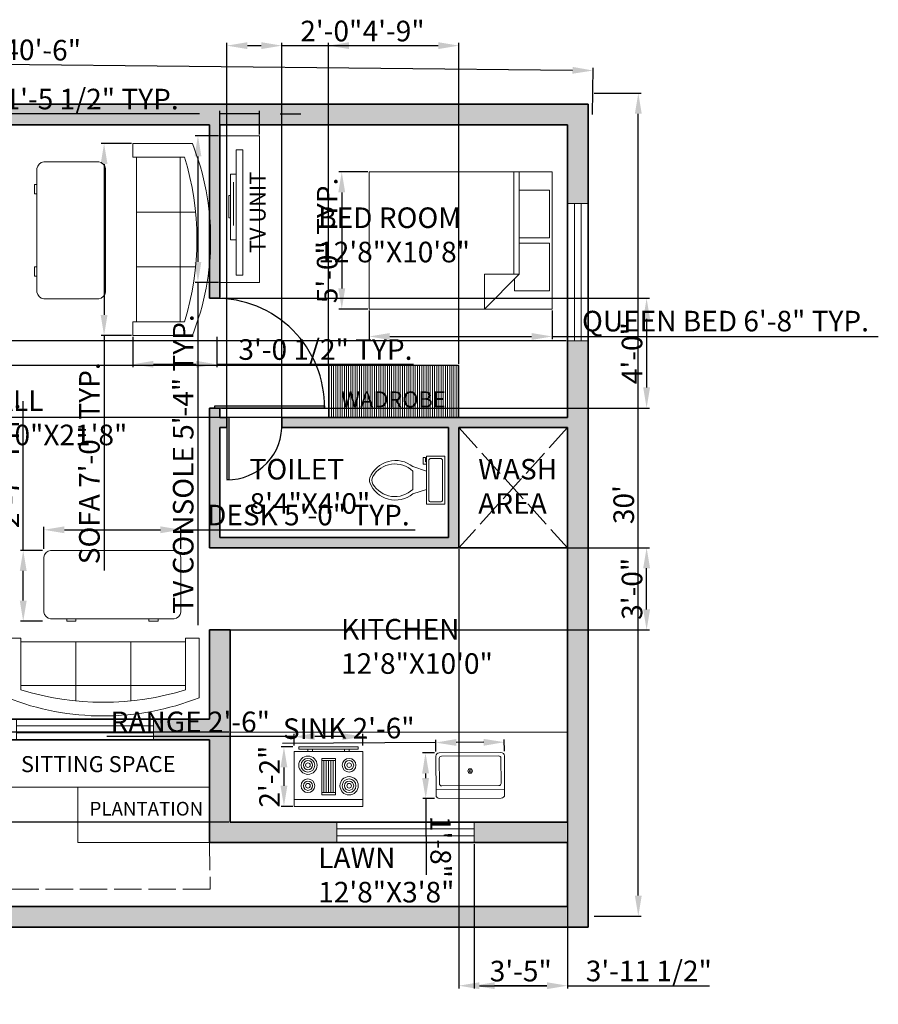
# Model space of a CAD drawing. Units: inches. Extents: x 33024 to 33675, y 11501 to 11939.
# Tile 3 of 3: x 33299 to 33675, y 11501 to 11932. Entities that reach past the tile are written whole.
import ezdxf

# ---------------------------------------------------------------- set-up
doc = ezdxf.new("R2010")
doc.units = ezdxf.units.IN
doc.linetypes.add('ACAD_ISO02W100', pattern=[15, 12, -3])
for name, color, linetype, lineweight in [('A-ANNO-DIMS', 2, 'Continuous', 18), ('A-ANNO-TEXT', 7, 'Continuous', 18), ('A-AREA-IDEN', 7, 'Continuous', 18), ('A-DOOR', 4, 'Continuous', 25), ('A-EQPM', 9, 'Continuous', 18), ('A-FLOR-FIXT', 9, 'Continuous', 18), ('A-FLOR-OPEN', 8, 'ACAD_ISO02W100', 13), ('A-FLOR-OVHD', 8, 'ACAD_ISO02W100', 13), ('A-FURN', 8, 'Continuous', 18), ('A-FURN-FIXD', 8, 'Continuous', 18), ('A-FURN-PATT', 252, 'Continuous', 9), ('A-GLAZ', 4, 'Continuous', 18), ('A-WALL', 7, 'Continuous', 35), ('L-PLNT', 3, 'Continuous', 18)]:
    doc.layers.add(name, color=color, linetype=linetype, lineweight=lineweight)
doc.layers.add('A-WALL-PATT', color=242, linetype='Continuous', lineweight=13, true_color=0xcd2027)
doc.styles.get("Standard").update_dxf_attribs({"font": 'arial.ttf'})
doc.dimstyles.new('ISO-25', dxfattribs={"dimtxt": 9, "dimasz": 9, "dimexe": 1.25, "dimexo": 0.625, "dimtad": 1, "dimdec": 1, "dimrnd": 9, "dimlunit": 3, "dimtxsty": 'Standard', "dimcen": 2.5, "dimadec": 0, "dimazin": 0, "dimtfac": 1, "dimtdec": 1, "dimtmove": 0, "dimatfit": 3, "dimfxl": 1, "dimarcsym": 0})

# ---------------------------------------------------------------- blocks, each defined once
blk = doc.blocks.new('Range-Oven - 30 in top')
for p, q in [((0, -3), (30, -3)), ((12, -6), (18, -6)), ((13, -20), (13, -6)), ((14, -6), (14, -20)), ((15, -20), (15, -6)), ((16, -6), (16, -20)), ((17, -20), (17, -6)), ((18, -20), (12, -20)), ((6, -24), (6, -25)), ((8, -25), (8, -24)), ((22, -25), (22, -24)), ((24, -24), (24, -25))]:
    blk.add_line(p, q)
for points in [[(0, -24), (0, 0), (30, 0), (30, -24)], [(12, -21), (12, -5), (18, -5), (18, -21)], [(2, -26), (2, -25), (28, -25), (28, -26)]]:
    blk.add_lwpolyline(points, close=True)
for centre, radius in [((6, -9), 4), ((6, -9), 3), ((6, -9), 2), ((6, -9), 1), ((24, -9), 3), ((24, -9), 2), ((24, -9), 1), ((6, -18), 3), ((6, -18), 2), ((6, -18), 1), ((24, -18), 4), ((24, -18), 3), ((24, -18), 2), ((24, -18), 1)]:
    blk.add_circle(centre, radius)
blk = doc.blocks.new('Sink-single - 30 in top')
blk.add_line((-15, -3.999996), (15, -3.999996))
for points in [[(-13.5, 0), (13.5, 0)], [(-15, -18.499996), (-15, -1.5)], [(15, -1.5), (15, -18.499996)], [(-13.5, -17.499996), (-13.5, -6.499996)], [(-12.5, -5.499996), (12.5, -5.499996)], [(13.5, -6.499996), (13.5, -17.499996)], [(13.5, -19.999996), (-13.5, -19.999996)], [(12.5, -18.499996), (-12.5, -18.499996)]]:
    blk.add_lwpolyline(points)
for radius in [1, 0.5]:
    blk.add_circle((0, -11.999996), radius)
for centre, radius, start, end in [((-13.5, -1.5), 1.5, 90, 180), ((13.5, -1.5), 1.5, 0, 90), ((-12.5, -6.499996), 1, 90, 180), ((12.5, -6.499996), 1, 0, 90), ((-13.5, -18.499996), 1.5, 180, 270), ((-12.5, -17.499996), 1, 180, 270), ((12.5, -17.499996), 1, 270, 0), ((13.5, -18.499996), 1.5, 270, 0)]:
    blk.add_arc(centre, radius, start, end)
blk = doc.blocks.new('Toilet - top')
for p, q in [((9.5, -6), (9.5, -2)), ((-10, -8.5), (-8, -8.5)), ((-10, -9.5), (-10, -8.5)), ((-8, -8.5), (-8, -8)), ((-7, -8), (-7, -9.5)), ((-4, -8), (-6, -14)), ((4, -8), (6, -14)), ((-7, -9.5), (-10, -9.5)), ((4, -14), (-4, -14))]:
    blk.add_line(p, q)
blk.add_lwpolyline([(10.5, -8), (10.5, 0), (-10.5, 0), (-10.5, -8)], close=True)
for points in [[(-9.5, -2), (-9.5, -6)], [(8.5, -1), (-8.5, -1)], [(-8.5, -7), (8.5, -7)]]:
    blk.add_lwpolyline(points)
for centre, radius, start, end in [((-8.62, -1.88), 0.884, 81.8699, 188.1301), ((8.62, -1.88), 0.884, 351.8699, 98.1301), ((-8.62, -6.12), 0.884, 171.8699, 278.1301), ((8.62, -6.12), 0.884, 261.8699, 8.1301), ((3.52, -21.58), 12.17, 141.4691, 247.9714), ((4.2, -21.82), 11.33, 136.3677, 238.9468), ((-3.52, -21.58), 12.17, 292.0284, 38.5307), ((-4.2, -21.82), 11.33, 301.053, 43.6321), ((0, -27.88), 4, 245.7318, 294.2682), ((0, -29), 4, 254.8605, 285.1395)]:
    blk.add_arc(centre, radius, start, end)
blk = doc.blocks.new('Bed - Queen')
for p, q in [((0, -80.00003), (0, 0)), ((0, 0), (59.99999, 0)), ((59.99999, 0), (59.99999, -80.00003)), ((7.99999, -1.2), (28.79998, -1.2)), ((7.99999, -14.4), (7.99999, -1.2)), ((28.79998, -1.2), (28.79998, -14.4)), ((31.19999, -1.2), (51.99999, -1.2)), ((31.19999, -14.4), (31.19999, -1.2)), ((51.99999, -1.2), (51.99999, -16.4)), ((0, -14.4), (44.8, -14.4)), ((44.8, -16.8), (0, -16.8)), ((59.99999, -29.6), (44.8, -14.4)), ((44.8, -14.4), (44.8, -29.6)), ((51.99999, -16.4), (46.79936, -16.4)), ((44.8, -29.6), (59.99999, -29.6)), ((59.99999, -80.00003), (0, -80.00003))]:
    blk.add_line(p, q)
blk = doc.blocks.new('Sofa - Roundback 7 ft.')
for p, q in [((-12.00002, -32.4421), (-12.00003, -6.5971)), ((11.99997, -32.4421), (11.99998, -6.5971)), ((-36.000027, -34), (-36.000027, -11.4696)), ((35.99998, -34), (35.99998, -11.4696)), ((-35.999844, -13.3819), (35.9998, -13.3819)), ((-36.000027, -32.4421), (35.99998, -32.4421))]:
    blk.add_line(p, q)
for points in [[(-36.000027, -34), (-42.000027, -34), (-42.000027, -8)], [(41.99998, -8), (41.99998, -34), (35.99998, -34)]]:
    blk.add_lwpolyline(points)
for centre, radius, start, end in [((0, -114.25), 114.25, 68.43141, 111.5686), ((-0.00001, -127.1968), 121.1968, 72.72033, 107.2797)]:
    blk.add_arc(centre, radius, start, end)
blk = doc.blocks.new('Desk - 30 x 60 in.')
for p, q in [((-26.999995, 0), (26.999995, 0)), ((-29.999995, -27), (-29.999995, -3)), ((29.999995, -3), (29.999995, -27)), ((26.999995, -30), (-26.999995, -30)), ((-20.000005, -30), (-20.000005, -31)), ((-16.000005, -31), (-16.000005, -30)), ((15.999995, -31), (15.999995, -30)), ((19.999995, -30), (19.999995, -31)), ((-20.000005, -31), (-16.000005, -31)), ((19.999995, -31), (15.999995, -31))]:
    blk.add_line(p, q)
for centre, start, end in [((-26.499995, -3.5), 98.1301, 171.8699), ((26.499995, -3.5), 8.130102, 81.8699), ((-26.499995, -26.5), 188.1301, 261.8699), ((26.499995, -26.5), 278.1301, 351.8699)]:
    blk.add_arc(centre, 3.535534, start, end)
blk = doc.blocks.new('*D8')
at = {"layer": 'A-ANNO-DIMS', "color": 0, "lineweight": -2, "transparency": 16777216}
for p, q in [((33068.04, 11895.8), (33068.26, 11916.32)), ((33077.25, 11914.97), (33541.21, 11909.99)), ((33550.01, 11890.62), (33550.23, 11911.14))]:
    blk.add_line(p, q, dxfattribs=at)
at = {"layer": 'A-ANNO-DIMS', "color": 0, "transparency": 16777216}
for points in [[(33077.26, 11916.47), (33077.23, 11913.47), (33068.25, 11915.07)], [(33541.23, 11911.49), (33541.2, 11908.49), (33550.21, 11909.89)]]:
    blk.add_solid(points, dxfattribs=at)
at = {"layer": 'Defpoints', "color": 0, "transparency": 16777216}
for p in [(33550.21, 11909.89), (33068.03, 11895.18), (33550, 11890)]:
    blk.add_point(p, dxfattribs=at)
at = {"layer": 'A-ANNO-DIMS', "color": 0, "transparency": 16777216, "insert": (33309.29, 11917.7), "char_height": 9, "attachment_point": 5, "rotation": 359.3847}
blk.add_mtext('40\'-6"', dxfattribs=at)
blk = doc.blocks.new('*D9')
at = {"layer": 'A-ANNO-DIMS', "color": 0, "lineweight": -2, "transparency": 16777216}
for p, q in [((33550.63, 11900), (33571.25, 11900)), ((33570, 11549), (33570, 11891)), ((33550.63, 11540), (33571.25, 11540))]:
    blk.add_line(p, q, dxfattribs=at)
at = {"layer": 'A-ANNO-DIMS', "color": 0, "transparency": 16777216}
for points in [[(33568.5, 11891), (33571.5, 11891), (33570, 11900)], [(33568.5, 11549), (33571.5, 11549), (33570, 11540)]]:
    blk.add_solid(points, dxfattribs=at)
at = {"layer": 'Defpoints', "color": 0, "transparency": 16777216}
for p in [(33550, 11900), (33570, 11900), (33550, 11540)]:
    blk.add_point(p, dxfattribs=at)
at = {"layer": 'A-ANNO-DIMS', "color": 0, "transparency": 16777216, "insert": (33564.78, 11720), "char_height": 9, "attachment_point": 5, "rotation": 90}
blk.add_mtext("30'", dxfattribs=at)
blk = doc.blocks.new('TV-CONSOLE-64')
for p, q in [((-17.33, 64.14), (-17.33, 0)), ((-7.13, 45.53), (-7.13, 45.53)), ((-7.13, 45.53), (-4.58, 45.53)), ((-4.58, 45.53), (-4.58, 16.72)), ((-5.92, 39.3), (-5.92, 20.26)), ((-4.58, 35.87), (-3.95, 35.87)), ((-3.95, 35.87), (-3.95, 26.18)), ((-3.95, 26.18), (-4.58, 26.18)), ((-4.58, 16.72), (-7.13, 16.72))]:
    blk.add_line(p, q)
blk.add_lwpolyline([(-17.33, 64.14), (0, 64.14), (0, 0), (-17.33, 0)])
blk.add_lwpolyline([(-10.08, 61), (-7.13, 61), (-7.13, 6.14), (-10.08, 6.14)], close=True)
blk = doc.blocks.new('WIN-60X9')
for p, q in [((0, 9), (0, 0)), ((60, 9), (60, 0)), ((60, 6), (0, 6)), ((60, 3), (0, 3))]:
    blk.add_line(p, q)
blk = doc.blocks.new('*D14')
at = {"layer": 'A-ANNO-DIMS', "color": 0, "lineweight": -2, "transparency": 16777216}
for p, q in [((33386.41, 11881.35), (33376.16, 11881.35)), ((33377.41, 11872.35), (33377.41, 11826.21)), ((33386.41, 11817.21), (33376.16, 11817.21)), ((33377.41, 11817.21), (33377.41, 11667.34))]:
    blk.add_line(p, q, dxfattribs=at)
at = {"layer": 'A-ANNO-DIMS', "color": 0, "transparency": 16777216}
for points in [[(33375.91, 11872.35), (33378.91, 11872.35), (33377.41, 11881.35)], [(33375.91, 11826.21), (33378.91, 11826.21), (33377.41, 11817.21)]]:
    blk.add_solid(points, dxfattribs=at)
at = {"layer": 'Defpoints', "color": 0, "transparency": 16777216}
for p in [(33387.03, 11881.35), (33377.41, 11817.21), (33387.03, 11817.21)]:
    blk.add_point(p, dxfattribs=at)
at = {"layer": 'A-ANNO-DIMS', "color": 0, "transparency": 16777216, "insert": (33372.13, 11737.78), "char_height": 9, "attachment_point": 5, "rotation": 90}
blk.add_mtext('TV CONSOLE 5\'-4" TYP.', dxfattribs=at)
blk = doc.blocks.new('*D15')
at = {"layer": 'A-ANNO-DIMS', "color": 0, "lineweight": -2, "transparency": 16777216}
for p, q in [((33387.03, 11881.98), (33387.03, 11892.22)), ((33404.36, 11881.98), (33404.36, 11892.22)), ((33378.03, 11890.97), (33292.8, 11890.97)), ((33404.36, 11890.97), (33387.03, 11890.97)), ((33413.36, 11890.97), (33422.36, 11890.97))]:
    blk.add_line(p, q, dxfattribs=at)
at = {"layer": 'A-ANNO-DIMS', "color": 0, "transparency": 16777216}
for points in [[(33378.03, 11892.47), (33378.03, 11889.47), (33387.03, 11890.97)], [(33413.36, 11892.47), (33413.36, 11889.47), (33404.36, 11890.97)]]:
    blk.add_solid(points, dxfattribs=at)
at = {"layer": 'Defpoints', "color": 0, "transparency": 16777216}
for p in [(33387.03, 11890.97), (33387.03, 11881.35), (33404.36, 11881.35)]:
    blk.add_point(p, dxfattribs=at)
at = {"layer": 'A-ANNO-DIMS', "color": 0, "transparency": 16777216, "insert": (33330.92, 11896.25), "char_height": 9, "attachment_point": 5}
blk.add_mtext('1\'-5 1/2" TYP.', dxfattribs=at)
blk = doc.blocks.new('*D18')
at = {"layer": 'A-ANNO-DIMS', "color": 0, "lineweight": -2, "transparency": 16777216}
for p, q in [((33452.31, 11804.94), (33452.31, 11792.32)), ((33532.31, 11804.94), (33532.31, 11792.32)), ((33461.31, 11793.57), (33523.31, 11793.57)), ((33532.31, 11793.57), (33674.95, 11793.57))]:
    blk.add_line(p, q, dxfattribs=at)
at = {"layer": 'A-ANNO-DIMS', "color": 0, "transparency": 16777216}
for points in [[(33461.31, 11795.07), (33461.31, 11792.07), (33452.31, 11793.57)], [(33523.31, 11795.07), (33523.31, 11792.07), (33532.31, 11793.57)]]:
    blk.add_solid(points, dxfattribs=at)
at = {"layer": 'Defpoints', "color": 0, "transparency": 16777216}
for p in [(33452.31, 11805.57), (33532.31, 11805.57), (33532.31, 11793.57)]:
    blk.add_point(p, dxfattribs=at)
at = {"layer": 'A-ANNO-DIMS', "color": 0, "transparency": 16777216, "insert": (33608.13, 11799.12), "char_height": 9, "attachment_point": 5}
blk.add_mtext('QUEEN BED 6\'-8" TYP.', dxfattribs=at)
blk = doc.blocks.new('*D19')
at = {"layer": 'A-ANNO-DIMS', "color": 0, "lineweight": -2, "transparency": 16777216}
for p, q in [((33451.69, 11865.57), (33439.06, 11865.57)), ((33440.31, 11856.57), (33440.31, 11814.57)), ((33451.69, 11805.57), (33439.06, 11805.57))]:
    blk.add_line(p, q, dxfattribs=at)
at = {"layer": 'A-ANNO-DIMS', "color": 0, "transparency": 16777216}
for points in [[(33438.81, 11856.57), (33441.81, 11856.57), (33440.31, 11865.57)], [(33438.81, 11814.57), (33441.81, 11814.57), (33440.31, 11805.57)]]:
    blk.add_solid(points, dxfattribs=at)
at = {"layer": 'Defpoints', "color": 0, "transparency": 16777216}
for p in [(33452.31, 11865.57), (33440.31, 11805.57), (33452.31, 11805.57)]:
    blk.add_point(p, dxfattribs=at)
at = {"layer": 'A-ANNO-DIMS', "color": 0, "transparency": 16777216, "insert": (33435.09, 11835.57), "char_height": 9, "attachment_point": 5, "rotation": 90}
blk.add_mtext('5\'-0" TYP.', dxfattribs=at)
blk = doc.blocks.new('*D20')
at = {"layer": 'A-ANNO-DIMS', "color": 0, "lineweight": -2, "transparency": 16777216}
for p, q in [((33348.34, 11878), (33335.12, 11878)), ((33336.37, 11869), (33336.37, 11803)), ((33348.34, 11794), (33335.12, 11794)), ((33336.37, 11794), (33336.37, 11691.21))]:
    blk.add_line(p, q, dxfattribs=at)
at = {"layer": 'A-ANNO-DIMS', "color": 0, "transparency": 16777216}
for points in [[(33334.87, 11869), (33337.87, 11869), (33336.37, 11878)], [(33334.87, 11803), (33337.87, 11803), (33336.37, 11794)]]:
    blk.add_solid(points, dxfattribs=at)
at = {"layer": 'Defpoints', "color": 0, "transparency": 16777216}
for p in [(33348.97, 11878), (33336.37, 11794), (33348.97, 11794)]:
    blk.add_point(p, dxfattribs=at)
at = {"layer": 'A-ANNO-DIMS', "color": 0, "transparency": 16777216, "insert": (33331.09, 11738.1), "char_height": 9, "attachment_point": 5, "rotation": 90}
blk.add_mtext('SOFA 7\'-0" TYP.', dxfattribs=at)
blk = doc.blocks.new('*D21')
at = {"layer": 'A-ANNO-DIMS', "color": 0, "lineweight": -2, "transparency": 16777216}
for p, q in [((33348.97, 11793.37), (33348.97, 11780.15)), ((33385.63, 11793.37), (33385.63, 11780.15)), ((33357.97, 11781.4), (33376.63, 11781.4)), ((33385.63, 11781.4), (33471.71, 11781.4))]:
    blk.add_line(p, q, dxfattribs=at)
at = {"layer": 'A-ANNO-DIMS', "color": 0, "transparency": 16777216}
for points in [[(33357.97, 11782.9), (33357.97, 11779.9), (33348.97, 11781.4)], [(33376.63, 11782.9), (33376.63, 11779.9), (33385.63, 11781.4)]]:
    blk.add_solid(points, dxfattribs=at)
at = {"layer": 'Defpoints', "color": 0, "transparency": 16777216}
for p in [(33348.97, 11794), (33385.63, 11794), (33385.63, 11781.4)]:
    blk.add_point(p, dxfattribs=at)
at = {"layer": 'A-ANNO-DIMS', "color": 0, "transparency": 16777216, "insert": (33433.17, 11786.68), "char_height": 9, "attachment_point": 5}
blk.add_mtext('3\'-0 1/2" TYP.', dxfattribs=at)
blk = doc.blocks.new('*D22')
at = {"layer": 'A-ANNO-DIMS', "color": 0, "lineweight": -2, "transparency": 16777216}
for p, q in [((33310, 11700.63), (33310, 11710.25)), ((33319, 11709), (33361, 11709)), ((33370, 11700.63), (33370, 11710.25)), ((33370, 11709), (33472.39, 11709))]:
    blk.add_line(p, q, dxfattribs=at)
at = {"layer": 'A-ANNO-DIMS', "color": 0, "transparency": 16777216}
for points in [[(33319, 11710.5), (33319, 11707.5), (33310, 11709)], [(33361, 11710.5), (33361, 11707.5), (33370, 11709)]]:
    blk.add_solid(points, dxfattribs=at)
at = {"layer": 'Defpoints', "color": 0, "transparency": 16777216}
for p in [(33370, 11709), (33310, 11700), (33370, 11700)]:
    blk.add_point(p, dxfattribs=at)
at = {"layer": 'A-ANNO-DIMS', "color": 0, "transparency": 16777216, "insert": (33425.7, 11714.28), "char_height": 9, "attachment_point": 5}
blk.add_mtext('DESK 5\'-0" TYP.', dxfattribs=at)
blk = doc.blocks.new('*D23')
at = {"layer": 'A-ANNO-DIMS', "color": 0, "lineweight": -2, "transparency": 16777216}
for p, q in [((33301, 11700), (33301, 11765.26)), ((33309.38, 11700), (33299.75, 11700)), ((33301, 11678), (33301, 11691)), ((33309.38, 11669), (33299.75, 11669))]:
    blk.add_line(p, q, dxfattribs=at)
at = {"layer": 'A-ANNO-DIMS', "color": 0, "transparency": 16777216}
for points in [[(33299.5, 11691), (33302.5, 11691), (33301, 11700)], [(33299.5, 11678), (33302.5, 11678), (33301, 11669)]]:
    blk.add_solid(points, dxfattribs=at)
at = {"layer": 'Defpoints', "color": 0, "transparency": 16777216}
for p in [(33301, 11700), (33310, 11700), (33310, 11669)]:
    blk.add_point(p, dxfattribs=at)
at = {"layer": 'A-ANNO-DIMS', "color": 0, "transparency": 16777216, "insert": (33295.85, 11737.13), "char_height": 9, "attachment_point": 5, "rotation": 90}
blk.add_mtext('2\'-7" TYP.', dxfattribs=at)
blk = doc.blocks.new('*D24')
at = {"layer": 'A-ANNO-DIMS', "color": 0, "lineweight": -2, "transparency": 16777216}
for p, q in [((33419.52, 11618.53), (33337.61, 11618.53)), ((33419.52, 11614.65), (33419.52, 11619.78)), ((33440.52, 11618.53), (33428.52, 11618.53)), ((33449.52, 11614.65), (33449.52, 11619.78))]:
    blk.add_line(p, q, dxfattribs=at)
at = {"layer": 'A-ANNO-DIMS', "color": 0, "transparency": 16777216}
for points in [[(33428.52, 11620.03), (33428.52, 11617.03), (33419.52, 11618.53)], [(33440.52, 11620.03), (33440.52, 11617.03), (33449.52, 11618.53)]]:
    blk.add_solid(points, dxfattribs=at)
at = {"layer": 'Defpoints', "color": 0, "transparency": 16777216}
for p in [(33419.52, 11618.53), (33419.52, 11614.03), (33449.52, 11614.03)]:
    blk.add_point(p, dxfattribs=at)
at = {"layer": 'A-ANNO-DIMS', "color": 0, "transparency": 16777216, "insert": (33374.06, 11623.81), "char_height": 9, "attachment_point": 5}
blk.add_mtext('RANGE 2\'-6"', dxfattribs=at)
blk = doc.blocks.new('*D25')
at = {"layer": 'A-ANNO-DIMS', "color": 0, "lineweight": -2, "transparency": 16777216}
for p, q in [((33418.89, 11614.03), (33413.77, 11614.03)), ((33415.02, 11605.03), (33415.02, 11597.03)), ((33418.89, 11588.03), (33413.77, 11588.03))]:
    blk.add_line(p, q, dxfattribs=at)
at = {"layer": 'A-ANNO-DIMS', "color": 0, "transparency": 16777216}
for points in [[(33413.52, 11605.03), (33416.52, 11605.03), (33415.02, 11614.03)], [(33413.52, 11597.03), (33416.52, 11597.03), (33415.02, 11588.03)]]:
    blk.add_solid(points, dxfattribs=at)
at = {"layer": 'Defpoints', "color": 0, "transparency": 16777216}
for p in [(33419.52, 11614.03), (33415.02, 11588.03), (33419.52, 11588.03)]:
    blk.add_point(p, dxfattribs=at)
at = {"layer": 'A-ANNO-DIMS', "color": 0, "transparency": 16777216, "insert": (33409.88, 11601.03), "char_height": 9, "attachment_point": 5, "rotation": 90}
blk.add_mtext('2\'-2"', dxfattribs=at)
blk = doc.blocks.new('*D26')
at = {"layer": 'A-ANNO-DIMS', "color": 0, "lineweight": -2, "transparency": 16777216}
for p, q in [((33481.4, 11615.92), (33414.43, 11615.55)), ((33481.42, 11612.05), (33481.39, 11617.17)), ((33502.4, 11616.04), (33490.4, 11615.97)), ((33511.42, 11612.21), (33511.39, 11617.34))]:
    blk.add_line(p, q, dxfattribs=at)
at = {"layer": 'A-ANNO-DIMS', "color": 0, "transparency": 16777216}
for points in [[(33490.39, 11617.47), (33490.41, 11614.47), (33481.4, 11615.92)], [(33502.39, 11617.54), (33502.41, 11614.54), (33511.4, 11616.09)]]:
    blk.add_solid(points, dxfattribs=at)
at = {"layer": 'Defpoints', "color": 0, "transparency": 16777216}
for p in [(33481.4, 11615.92), (33511.42, 11611.59), (33481.42, 11611.42)]:
    blk.add_point(p, dxfattribs=at)
at = {"layer": 'A-ANNO-DIMS', "color": 0, "transparency": 16777216, "insert": (33443.38, 11620.99), "char_height": 9, "attachment_point": 5, "rotation": 0.3185}
blk.add_mtext('SINK 2\'-6"', dxfattribs=at)
blk = doc.blocks.new('*D27')
at = {"layer": 'A-ANNO-DIMS', "color": 0, "lineweight": -2, "transparency": 16777216}
for p, q in [((33480.8, 11611.42), (33475.67, 11611.39)), ((33476.97, 11602.4), (33476.98, 11600.4)), ((33480.91, 11591.42), (33475.78, 11591.39)), ((33477.03, 11591.4), (33477.22, 11558.07))]:
    blk.add_line(p, q, dxfattribs=at)
at = {"layer": 'A-ANNO-DIMS', "color": 0, "transparency": 16777216}
for points in [[(33478.47, 11602.41), (33475.47, 11602.39), (33476.92, 11611.4)], [(33478.48, 11600.41), (33475.48, 11600.39), (33477.03, 11591.4)]]:
    blk.add_solid(points, dxfattribs=at)
at = {"layer": 'Defpoints', "color": 0, "transparency": 16777216}
for p in [(33481.42, 11611.42), (33477.03, 11591.4), (33481.53, 11591.42)]:
    blk.add_point(p, dxfattribs=at)
at = {"layer": 'A-ANNO-DIMS', "color": 0, "transparency": 16777216, "insert": (33482.37, 11570.26), "char_height": 9, "attachment_point": 5, "rotation": 270.3185}
blk.add_mtext('1\'-8"', dxfattribs=at)
blk = doc.blocks.new('*D31')
at = {"layer": 'A-ANNO-DIMS', "color": 0, "lineweight": -2, "transparency": 16777216}
for p, q in [((33042.43, 11791.72), (33042.43, 11847.01)), ((33538.41, 11791.72), (33041.18, 11791.72)), ((33042.43, 11767.18), (33042.43, 11782.72)), ((33538.41, 11758.18), (33041.18, 11758.18))]:
    blk.add_line(p, q, dxfattribs=at)
at = {"layer": 'A-ANNO-DIMS', "color": 0, "transparency": 16777216}
for points in [[(33040.93, 11782.72), (33043.93, 11782.72), (33042.43, 11791.72)], [(33040.93, 11767.18), (33043.93, 11767.18), (33042.43, 11758.18)]]:
    blk.add_solid(points, dxfattribs=at)
at = {"layer": 'Defpoints', "color": 0, "transparency": 16777216}
for p in [(33042.43, 11791.72), (33539.03, 11791.72), (33539.03, 11758.18)]:
    blk.add_point(p, dxfattribs=at)
at = {"layer": 'A-ANNO-DIMS', "color": 0, "transparency": 16777216, "insert": (33037.15, 11823.87), "char_height": 9, "attachment_point": 5, "rotation": 90}
blk.add_mtext('2\'-9 1/2"', dxfattribs=at)
blk = doc.blocks.new('*D32')
at = {"layer": 'A-ANNO-DIMS', "color": 0, "lineweight": -2, "transparency": 16777216}
for p, q in [((33498.14, 11571.55), (33498.14, 11508.33)), ((33539.03, 11571.55), (33539.03, 11508.33)), ((33530.03, 11509.58), (33507.14, 11509.58))]:
    blk.add_line(p, q, dxfattribs=at)
at = {"layer": 'A-ANNO-DIMS', "color": 0, "transparency": 16777216}
for points in [[(33507.14, 11511.08), (33507.14, 11508.08), (33498.14, 11509.58)], [(33530.03, 11511.08), (33530.03, 11508.08), (33539.03, 11509.58)]]:
    blk.add_solid(points, dxfattribs=at)
at = {"layer": 'Defpoints', "color": 0, "transparency": 16777216}
for p in [(33498.14, 11572.18), (33539.03, 11572.18), (33498.14, 11509.58)]:
    blk.add_point(p, dxfattribs=at)
at = {"layer": 'A-ANNO-DIMS', "color": 0, "transparency": 16777216, "insert": (33518.59, 11514.8), "char_height": 9, "attachment_point": 5}
blk.add_mtext('3\'-5"', dxfattribs=at)
blk = doc.blocks.new('*D36')
at = {"layer": 'A-ANNO-DIMS', "color": 0, "lineweight": -2, "transparency": 16777216}
for p, q in [((33387.66, 11810.27), (33574.88, 11810.27)), ((33573.63, 11801.27), (33573.63, 11771.27)), ((33387.66, 11762.27), (33574.88, 11762.27))]:
    blk.add_line(p, q, dxfattribs=at)
at = {"layer": 'A-ANNO-DIMS', "color": 0, "transparency": 16777216}
for points in [[(33572.13, 11801.27), (33575.13, 11801.27), (33573.63, 11810.27)], [(33572.13, 11771.27), (33575.13, 11771.27), (33573.63, 11762.27)]]:
    blk.add_solid(points, dxfattribs=at)
at = {"layer": 'Defpoints', "color": 0, "transparency": 16777216}
for p in [(33387.03, 11810.27), (33387.03, 11762.27), (33573.63, 11762.27)]:
    blk.add_point(p, dxfattribs=at)
at = {"layer": 'A-ANNO-DIMS', "color": 0, "transparency": 16777216, "insert": (33568.41, 11786.27), "char_height": 9, "attachment_point": 5, "rotation": 90}
blk.add_mtext('4\'-0"', dxfattribs=at)
blk = doc.blocks.new('*D38')
at = {"layer": 'A-ANNO-DIMS', "color": 0, "lineweight": -2, "transparency": 16777216}
for p, q in [((33390.07, 11754.3), (33390.07, 11922.03)), ((33414.07, 11754.3), (33414.07, 11922.03)), ((33399.07, 11920.78), (33405.07, 11920.78)), ((33414.07, 11920.78), (33448.4, 11920.78))]:
    blk.add_line(p, q, dxfattribs=at)
at = {"layer": 'A-ANNO-DIMS', "color": 0, "transparency": 16777216}
for points in [[(33399.07, 11922.28), (33399.07, 11919.28), (33390.07, 11920.78)], [(33405.07, 11922.28), (33405.07, 11919.28), (33414.07, 11920.78)]]:
    blk.add_solid(points, dxfattribs=at)
at = {"layer": 'Defpoints', "color": 0, "transparency": 16777216}
for p in [(33414.07, 11920.78), (33390.07, 11753.68), (33414.07, 11753.68)]:
    blk.add_point(p, dxfattribs=at)
at = {"layer": 'A-ANNO-DIMS', "color": 0, "transparency": 16777216, "insert": (33435.73, 11926), "char_height": 9, "attachment_point": 5}
blk.add_mtext('2\'-0"', dxfattribs=at)
blk = doc.blocks.new('*D39')
at = {"layer": 'A-ANNO-DIMS', "color": 0, "lineweight": -2, "transparency": 16777216}
for p, q in [((33383.16, 11701.18), (33574.88, 11701.18)), ((33573.63, 11674.18), (33573.63, 11692.18)), ((33383.16, 11665.18), (33574.88, 11665.18))]:
    blk.add_line(p, q, dxfattribs=at)
at = {"layer": 'A-ANNO-DIMS', "color": 0, "transparency": 16777216}
for points in [[(33572.13, 11692.18), (33575.13, 11692.18), (33573.63, 11701.18)], [(33572.13, 11674.18), (33575.13, 11674.18), (33573.63, 11665.18)]]:
    blk.add_solid(points, dxfattribs=at)
at = {"layer": 'Defpoints', "color": 0, "transparency": 16777216}
for p in [(33382.53, 11701.18), (33573.63, 11701.18), (33382.53, 11665.18)]:
    blk.add_point(p, dxfattribs=at)
at = {"layer": 'A-ANNO-DIMS', "color": 0, "transparency": 16777216, "insert": (33568.41, 11683.18), "char_height": 9, "attachment_point": 5, "rotation": 90}
blk.add_mtext('3\'-0"', dxfattribs=at)
blk = doc.blocks.new('*D45')
at = {"layer": 'A-ANNO-DIMS', "color": 0, "lineweight": -2, "transparency": 16777216}
for p, q in [((33434.44, 11781.52), (33434.44, 11922.03)), ((33491.54, 11781.52), (33491.54, 11922.03)), ((33443.44, 11920.78), (33482.54, 11920.78))]:
    blk.add_line(p, q, dxfattribs=at)
at = {"layer": 'A-ANNO-DIMS', "color": 0, "transparency": 16777216}
for points in [[(33443.44, 11922.28), (33443.44, 11919.28), (33434.44, 11920.78)], [(33482.54, 11922.28), (33482.54, 11919.28), (33491.54, 11920.78)]]:
    blk.add_solid(points, dxfattribs=at)
at = {"layer": 'Defpoints', "color": 0, "transparency": 16777216}
for p in [(33491.54, 11920.78), (33434.44, 11780.89), (33491.54, 11780.89)]:
    blk.add_point(p, dxfattribs=at)
at = {"layer": 'A-ANNO-DIMS', "color": 0, "transparency": 16777216, "insert": (33462.99, 11926), "char_height": 9, "attachment_point": 5}
blk.add_mtext('4\'-9"', dxfattribs=at)
blk = doc.blocks.new('*D46')
at = {"layer": 'A-ANNO-DIMS', "color": 0, "lineweight": -2, "transparency": 16777216}
for p, q in [((33042.43, 11780.89), (33042.43, 11842.18)), ((33490.92, 11780.89), (33041.18, 11780.89)), ((33042.43, 11767.18), (33042.43, 11771.89)), ((33490.92, 11758.18), (33041.18, 11758.18))]:
    blk.add_line(p, q, dxfattribs=at)
at = {"layer": 'A-ANNO-DIMS', "color": 0, "transparency": 16777216}
for points in [[(33040.93, 11771.89), (33043.93, 11771.89), (33042.43, 11780.89)], [(33040.93, 11767.18), (33043.93, 11767.18), (33042.43, 11758.18)]]:
    blk.add_solid(points, dxfattribs=at)
at = {"layer": 'Defpoints', "color": 0, "transparency": 16777216}
for p in [(33042.43, 11780.89), (33491.54, 11780.89), (33491.54, 11758.18)]:
    blk.add_point(p, dxfattribs=at)
at = {"layer": 'A-ANNO-DIMS', "color": 0, "transparency": 16777216, "insert": (33037.15, 11816.04), "char_height": 9, "attachment_point": 5, "rotation": 90}
blk.add_mtext('1\'-10 1/2"', dxfattribs=at)
blk = doc.blocks.new('*D47')
at = {"layer": 'A-ANNO-DIMS', "color": 0, "lineweight": -2, "transparency": 16777216}
for p, q in [((33491.53, 11700.55), (33491.53, 11508.33)), ((33539.03, 11700.55), (33539.03, 11508.33)), ((33500.53, 11509.58), (33530.03, 11509.58)), ((33539.03, 11509.58), (33601.16, 11509.58))]:
    blk.add_line(p, q, dxfattribs=at)
at = {"layer": 'A-ANNO-DIMS', "color": 0, "transparency": 16777216}
for points in [[(33500.53, 11511.08), (33500.53, 11508.08), (33491.53, 11509.58)], [(33530.03, 11511.08), (33530.03, 11508.08), (33539.03, 11509.58)]]:
    blk.add_solid(points, dxfattribs=at)
at = {"layer": 'Defpoints', "color": 0, "transparency": 16777216}
for p in [(33491.53, 11701.18), (33539.03, 11701.18), (33539.03, 11509.58)]:
    blk.add_point(p, dxfattribs=at)
at = {"layer": 'A-ANNO-DIMS', "color": 0, "transparency": 16777216, "insert": (33574.6, 11514.86), "char_height": 9, "attachment_point": 5}
blk.add_mtext('3\'-11 1/2"', dxfattribs=at)
blk = doc.blocks.new('*D48')
at = {"layer": 'A-ANNO-DIMS', "color": 0, "lineweight": -2, "transparency": 16777216}
for p, q in [((33042.43, 11620.53), (33042.43, 11675.67)), ((33390.91, 11620.53), (33041.18, 11620.53)), ((33042.43, 11590.18), (33042.43, 11611.53)), ((33390.91, 11581.18), (33041.18, 11581.18))]:
    blk.add_line(p, q, dxfattribs=at)
at = {"layer": 'A-ANNO-DIMS', "color": 0, "transparency": 16777216}
for points in [[(33040.93, 11611.53), (33043.93, 11611.53), (33042.43, 11620.53)], [(33040.93, 11590.18), (33043.93, 11590.18), (33042.43, 11581.18)]]:
    blk.add_solid(points, dxfattribs=at)
at = {"layer": 'Defpoints', "color": 0, "transparency": 16777216}
for p in [(33042.43, 11620.53), (33391.53, 11620.53), (33391.53, 11581.18)]:
    blk.add_point(p, dxfattribs=at)
at = {"layer": 'A-ANNO-DIMS', "color": 0, "transparency": 16777216, "insert": (33037.15, 11652.6), "char_height": 9, "attachment_point": 5, "rotation": 90}
blk.add_mtext('3\'-3 1/2"', dxfattribs=at)

msp = doc.modelspace()

# ---------------------------------------------------------------- hatches: boundary and pattern name
at = {"layer": 'A-FURN-PATT'}
h = msp.add_hatch(dxfattribs=at)
h.set_pattern_fill('ANSI31', color=256, scale=0.29606299, angle=45, style=0)
h.paths.add_polyline_path([(33434.44, 11758.18), (33491.54, 11758.18), (33491.54, 11780.89), (33434.44, 11780.89)])
at = {"layer": 'A-WALL-PATT'}
h = msp.add_hatch(color=256, dxfattribs=at)
h.dxf.hatch_style = 1
h.paths.add_polyline_path([(33548.03, 11895.18), (33068.03, 11895.18), (33068.03, 11851.93), (33077.03, 11851.93), (33077.03, 11886.18), (33221.03, 11886.18), (33221.03, 11794.32, -0.012093), (33223.28, 11794.3), (33225.53, 11794.3), (33225.53, 11886.18), (33382.53, 11886.18), (33382.53, 11845.96, -0.043682), (33382.53, 11826.04), (33382.53, 11810.27), (33384.78, 11810.27, -0.005263), (33385.78, 11810.27), (33387.03, 11810.27), (33387.03, 11886.18), (33539.03, 11886.18), (33539.03, 11851.72), (33548.03, 11851.72)])
h.paths.add_polyline_path([(33077.03, 11791.93), (33068.03, 11791.93), (33068.03, 11535.18), (33077.03, 11535.18), (33077.03, 11544.18), (33077.03, 11737.68), (33116.53, 11737.68), (33116.53, 11685.18), (33221.03, 11685.18), (33221.03, 11617.18), (33228.7, 11617.18), (33228.7, 11626.18), (33225.53, 11626.18), (33225.53, 11746.3), (33221.03, 11746.3), (33221.03, 11742.18), (33215.96, 11742.18), (33215.96, 11737.68), (33221.03, 11737.68), (33221.03, 11689.68), (33121.03, 11689.68), (33121.03, 11737.68), (33179.96, 11737.68), (33191.96, 11737.68), (33191.96, 11738.93, -0.010637), (33191.96, 11739.93), (33191.96, 11742.18), (33179.96, 11742.18), (33077.03, 11742.18)])
h.paths.add_polyline_path([(33548.03, 11791.72), (33539.03, 11791.72), (33539.03, 11758.18), (33426.07, 11758.18), (33414.07, 11758.18), (33414.07, 11755.93, -0.023906), (33414.1, 11753.68), (33426.07, 11753.68), (33487.03, 11753.68), (33487.03, 11705.68), (33387.03, 11705.68), (33387.03, 11753.68), (33390.07, 11753.68), (33390.07, 11754.93), (33390.07, 11755.93), (33390.07, 11758.18), (33387.03, 11758.18), (33387.03, 11762.27), (33382.53, 11762.27), (33382.53, 11701.18), (33387.03, 11701.18), (33491.53, 11701.18), (33491.53, 11753.68), (33539.03, 11753.68), (33539.03, 11581.18), (33498.14, 11581.18), (33498.14, 11572.18), (33539.03, 11572.18), (33539.03, 11544.18), (33280.53, 11544.18), (33280.53, 11535.18), (33548.03, 11535.18)])
h.paths.add_polyline_path([(33391.53, 11626.18), (33391.53, 11626.18), (33391.53, 11665.18), (33382.53, 11665.18), (33382.53, 11626.18), (33358.03, 11626.18), (33358.03, 11617.18), (33382.53, 11617.18), (33382.53, 11572.18), (33387.03, 11572.18), (33438.14, 11572.18), (33438.14, 11581.18), (33391.53, 11581.18), (33391.53, 11614.89)], flags=17)

# ---------------------------------------------------------------- linework, layer by layer
at = {"layer": 'A-DOOR'}
for p, q in [((33384.78, 11762.27), (33384.78, 11763.27)), ((33384.78, 11763.27), (33432.78, 11763.27)), ((33432.78, 11762.27), (33387.03, 11762.27)), ((33432.78, 11763.27), (33432.78, 11762.27)), ((33391.07, 11758.18), (33390.07, 11758.18)), ((33391.07, 11730.93), (33391.07, 11758.18)), ((33390.07, 11755.93), (33390.07, 11754.93)), ((33390.07, 11754.93), (33390.07, 11730.93)), ((33390.07, 11730.93), (33391.07, 11730.93))]:
    msp.add_line(p, q, dxfattribs=at)
for centre, radius, start, end in [((33385.28, 11762.77), 47.5, 359.3969, 90.6031), ((33390.57, 11754.47), 23.55, 268.7832, 3.5551)]:
    msp.add_arc(centre, radius, start, end, dxfattribs=at)
at = {"layer": 'A-FLOR-OPEN'}
for p, q in [((33539.03, 11753.68), (33491.53, 11701.18)), ((33491.53, 11753.68), (33539.03, 11701.18))]:
    msp.add_line(p, q, dxfattribs=at)
at = {"layer": 'A-FLOR-OVHD'}
for p, q in [((33382.53, 11572.18), (33382.77, 11551.78)), ((33382.77, 11551.78), (33077.03, 11551.78))]:
    msp.add_line(p, q, dxfattribs=at)
at = {"layer": 'A-FURN-FIXD'}
for p, q in [((33434.44, 11780.89), (33491.54, 11780.89)), ((33434.44, 11758.18), (33434.44, 11780.89)), ((33491.54, 11758.18), (33491.54, 11780.89)), ((33391.53, 11620.53), (33539.03, 11620.53)), ((33278.11, 11596.48), (33382.53, 11596.48))]:
    msp.add_line(p, q, dxfattribs=at)
at = {"layer": 'A-WALL'}
for p, q in [((33548.03, 11895.18), (33068.03, 11895.18)), ((33548.03, 11535.18), (33548.03, 11895.18)), ((33382.53, 11886.18), (33225.53, 11886.18)), ((33382.53, 11810.27), (33382.53, 11886.18)), ((33539.03, 11886.18), (33387.03, 11886.18)), ((33387.03, 11810.27), (33387.03, 11886.18)), ((33539.03, 11758.18), (33539.03, 11886.18)), ((33382.53, 11810.27), (33387.03, 11810.27)), ((33382.53, 11701.18), (33382.53, 11762.27)), ((33382.53, 11762.27), (33387.03, 11762.27)), ((33387.03, 11758.18), (33387.03, 11762.27)), ((33390.07, 11758.18), (33387.03, 11758.18)), ((33390.07, 11758.18), (33390.07, 11753.68)), ((33426.07, 11758.18), (33414.07, 11758.18)), ((33414.07, 11758.18), (33414.07, 11753.68)), ((33539.03, 11758.18), (33426.07, 11758.18)), ((33387.03, 11705.68), (33387.03, 11753.68)), ((33390.07, 11753.68), (33387.03, 11753.68)), ((33414.07, 11753.68), (33426.07, 11753.68)), ((33487.03, 11753.68), (33426.07, 11753.68)), ((33487.03, 11705.68), (33487.03, 11753.68)), ((33539.03, 11753.68), (33491.53, 11753.68)), ((33491.53, 11701.18), (33491.53, 11753.68)), ((33539.03, 11581.18), (33539.03, 11753.68)), ((33487.03, 11705.68), (33387.03, 11705.68)), ((33387.03, 11701.18), (33382.53, 11701.18)), ((33539.03, 11701.18), (33387.03, 11701.18)), ((33382.53, 11626.18), (33382.53, 11665.18)), ((33391.53, 11665.18), (33382.53, 11665.18)), ((33391.53, 11665.18), (33391.53, 11626.18)), ((33382.53, 11626.18), (33276.7, 11626.18)), ((33391.53, 11614.89), (33391.53, 11626.18)), ((33391.53, 11626.18), (33391.53, 11626.18)), ((33382.53, 11617.18), (33221.03, 11617.18)), ((33382.53, 11617.18), (33382.53, 11572.18)), ((33391.53, 11614.89), (33391.53, 11581.18)), ((33539.03, 11581.18), (33391.53, 11581.18)), ((33382.53, 11572.18), (33387.03, 11572.18)), ((33539.03, 11572.18), (33387.03, 11572.18)), ((33539.03, 11544.18), (33539.03, 11572.18)), ((33280.53, 11544.18), (33539.03, 11544.18)), ((33068.03, 11535.18), (33548.03, 11535.18))]:
    msp.add_line(p, q, dxfattribs=at)
at = {"layer": 'L-PLNT'}
for p, q in [((33324.83, 11596.48), (33324.83, 11572.18)), ((33324.83, 11572.18), (33382.53, 11572.18))]:
    msp.add_line(p, q, dxfattribs=at)

# ---------------------------------------------------------------- block references
at = {"layer": 'A-EQPM', "rotation": 180}
msp.add_blockref('Range-Oven - 30 in top', (33449.52, 11588.03), dxfattribs=at)
at = {"layer": 'A-FLOR-FIXT'}
for name, p, rotation in [('Toilet - top', (33485.39, 11730.66), 270), ('Sink-single - 30 in top', (33496.53, 11591.51), 180.3184658995135)]:
    msp.add_blockref(name, p, dxfattribs=dict(at, rotation=rotation))
at = {"layer": 'A-FURN'}
for name, p, rotation in [('Sofa - Roundback 7 ft.', (33382.97, 11836), 270), ('Desk - 30 x 60 in.', (33337, 11840), 270), ('Bed - Queen', (33532.31, 11865.57), 270), ('Sofa - Roundback 7 ft.', (33336, 11627.56), 180)]:
    msp.add_blockref(name, p, dxfattribs=dict(at, rotation=rotation))
msp.add_blockref('Desk - 30 x 60 in.', (33340, 11700), dxfattribs=at)
at = {"layer": 'A-FURN-FIXD', "rotation": 180}
msp.add_blockref('TV-CONSOLE-64', (33387.03, 11881.35), dxfattribs=at)
at = {"layer": 'A-GLAZ', "rotation": 269.9999999999856}
msp.add_blockref('WIN-60X9', (33539.03, 11851.72), dxfattribs=at)
at = {"layer": 'A-GLAZ'}
for p in [(33298.03, 11617.18), (33438.14, 11572.18)]:
    msp.add_blockref('WIN-60X9', p, dxfattribs=at)

# ---------------------------------------------------------------- texts
at = {"layer": 'A-ANNO-TEXT', "insert": (33400, 11830), "char_height": 7, "attachment_point": 1, "rotation": 90}
msp.add_mtext_dynamic_manual_height_columns('TV UNIT', width=70, gutter_width=12.5, heights=[0], dxfattribs=at)
at = {"layer": 'A-ANNO-TEXT', "attachment_point": 1}
for s, width, insert, char_height in [('WADROBE', 70, (33439.95, 11769.53), 7), ('SITTING SPACE', 73.7349, (33300, 11610), 7), ('PLANTATION', 70, (33330, 11590), 6)]:
    msp.add_mtext_dynamic_manual_height_columns(s, width=width, gutter_width=12.5, heights=[0], dxfattribs=dict(at, insert=insert, char_height=char_height))
at = {"layer": 'A-AREA-IDEN', "char_height": 9, "attachment_point": 1}
for s, insert in [('BED ROOM\\P12\'8"X10\'8"', (33430, 11850)), ('HALL\\P14\'0"X21\'8"', (33280.14, 11769.99)), ('TOILET\\P8\'4"X4\'0"', (33400, 11740)), ('WASH\\PAREA', (33500, 11740)), ('KITCHEN\\P12\'8"X10\'0"', (33440, 11670)), ('LAWN\\P12\'8"X3\'8"', (33430, 11570))]:
    msp.add_mtext_dynamic_manual_height_columns(s, width=70, gutter_width=12.5, heights=[0], dxfattribs=dict(at, insert=insert))

# ---------------------------------------------------------------- dimensions: what is measured, and where the dimension line sits
at = {"layer": 'A-ANNO-DIMS'}
for base, p1, p2, picture, middle in [((33414.07, 11920.78), (33390.07, 11753.68), (33414.07, 11753.68), '*D38', (33435.73, 11926)), ((33491.54, 11920.78), (33434.44, 11780.89), (33491.54, 11780.89), '*D45', (33462.99, 11926)), ((33539.03, 11509.58), (33491.53, 11701.18), (33539.03, 11701.18), '*D47', (33574.6, 11514.86)), ((33498.14, 11509.58), (33539.03, 11572.18), (33498.14, 11572.18), '*D32', (33518.59, 11514.8))]:
    dim = msp.add_linear_dim(base=base, p1=p1, p2=p2, dimstyle='ISO-25', override={"dimdec": 1, "dimlfac": 1, "dimrnd": 0, "dimzin": 1, "dimdsep": 46, "dimlunit": 4, "dimfrac": 2}, dxfattribs=at)
    dim.commit()
    dim.dimension.update_dxf_attribs({"geometry": picture, "text_midpoint": middle})
dim = msp.add_aligned_dim(p1=(33068.03, 11895.18), p2=(33550, 11890), distance=19.89, dimstyle='ISO-25', override={"dimclrd": 0, "dimclre": 0, "dimclrt": 0}, dxfattribs=at)
dim.commit()
dim.dimension.update_dxf_attribs({"geometry": '*D8', "text_midpoint": (33309.29, 11917.7)})
for base, p1, p2, angle, text, picture, middle in [((33387.03, 11890.97), (33404.36, 11881.35), (33387.03, 11881.35), 180, '<> TYP.', '*D15', (33330.92, 11896.25)), ((33377.41, 11817.21), (33387.03, 11881.35), (33387.03, 11817.21), 270, 'TV CONSOLE <> TYP.', '*D14', (33372.13, 11737.78)), ((33336.37, 11794), (33348.97, 11878), (33348.97, 11794), 270, 'SOFA <> TYP.', '*D20', (33331.09, 11738.1)), ((33440.31, 11805.57), (33452.31, 11865.57), (33452.31, 11805.57), 270, '<> TYP.', '*D19', (33435.09, 11835.57)), ((33301, 11700), (33310, 11669), (33310, 11700), 90, '<> TYP.', '*D23', (33295.85, 11737.13)), ((33419.52, 11618.53), (33449.52, 11614.03), (33419.52, 11614.03), 180, 'RANGE <>', '*D24', (33374.06, 11623.81)), ((33481.4, 11615.92), (33511.42, 11611.59), (33481.42, 11611.42), 180.3185, 'SINK <>', '*D26', (33443.38, 11620.99))]:
    dim = msp.add_linear_dim(base=base, p1=p1, p2=p2, angle=angle, text=text, dimstyle='ISO-25', override={"dimdec": 1, "dimlfac": 1, "dimrnd": 0, "dimzin": 1, "dimdsep": 46, "dimlunit": 4, "dimfrac": 2}, dxfattribs=at)
    dim.commit()
    dim.dimension.update_dxf_attribs({"geometry": picture, "text_midpoint": middle})
for base, p1, p2, angle, override, picture, middle in [((33570, 11900), (33550, 11540), (33550, 11900), 90, {"dimclrd": 0, "dimclre": 0, "dimclrt": 0}, '*D9', (33564.78, 11720)), ((33042.43, 11791.72), (33539.03, 11758.18), (33539.03, 11791.72), 90, {"dimdec": 1, "dimlfac": 1, "dimrnd": 0, "dimzin": 1, "dimdsep": 46, "dimlunit": 4, "dimfrac": 2}, '*D31', (33037.15, 11823.87)), ((33042.43, 11780.89), (33491.54, 11758.18), (33491.54, 11780.89), 90, {"dimdec": 1, "dimlfac": 1, "dimrnd": 0, "dimzin": 1, "dimdsep": 46, "dimlunit": 4, "dimfrac": 2}, '*D46', (33037.15, 11816.04)), ((33573.63, 11762.27), (33387.03, 11810.27), (33387.03, 11762.27), 90, {"dimdec": 1, "dimlfac": 1, "dimrnd": 0, "dimzin": 1, "dimdsep": 46, "dimlunit": 4, "dimfrac": 2}, '*D36', (33568.41, 11786.27)), ((33573.63, 11701.18), (33382.53, 11665.18), (33382.53, 11701.18), 90, {"dimdec": 1, "dimlfac": 1, "dimrnd": 0, "dimzin": 1, "dimdsep": 46, "dimlunit": 4, "dimfrac": 2}, '*D39', (33568.41, 11683.18)), ((33042.4322, 11620.5337), (33391.5322, 11581.1761), (33391.5322, 11620.5337), 90, {"dimdec": 1, "dimlfac": 1, "dimrnd": 0, "dimzin": 1, "dimdsep": 46, "dimlunit": 4, "dimfrac": 2}, '*D48', (33037.1507, 11652.6034)), ((33415.02, 11588.03), (33419.52, 11614.03), (33419.52, 11588.03), 270, {"dimdec": 1, "dimlfac": 1, "dimrnd": 0, "dimzin": 1, "dimdsep": 46, "dimlunit": 4, "dimfrac": 2}, '*D25', (33409.88, 11601.03)), ((33477.03, 11591.4), (33481.42, 11611.42), (33481.53, 11591.42), 270.3185, {"dimdec": 1, "dimlfac": 1, "dimrnd": 0, "dimzin": 1, "dimdsep": 46, "dimlunit": 4, "dimfrac": 2}, '*D27', (33482.37, 11570.26))]:
    dim = msp.add_linear_dim(base=base, p1=p1, p2=p2, angle=angle, dimstyle='ISO-25', override=override, dxfattribs=at)
    dim.commit()
    dim.dimension.update_dxf_attribs({"geometry": picture, "text_midpoint": middle})
for base, p1, p2, text, picture, middle in [((33532.31, 11793.57), (33452.31, 11805.57), (33532.31, 11805.57), 'QUEEN BED <> TYP.', '*D18', (33608.13, 11799.12)), ((33385.63, 11781.4), (33348.97, 11794), (33385.63, 11794), '<> TYP.', '*D21', (33433.17, 11786.68)), ((33370, 11709), (33310, 11700), (33370, 11700), 'DESK <> TYP.', '*D22', (33425.7, 11714.28))]:
    dim = msp.add_linear_dim(base=base, p1=p1, p2=p2, text=text, dimstyle='ISO-25', override={"dimdec": 1, "dimlfac": 1, "dimrnd": 0, "dimzin": 1, "dimdsep": 46, "dimlunit": 4, "dimfrac": 2}, dxfattribs=at)
    dim.commit()
    dim.dimension.update_dxf_attribs({"geometry": picture, "text_midpoint": middle})

doc.saveas('drawing.dxf')
